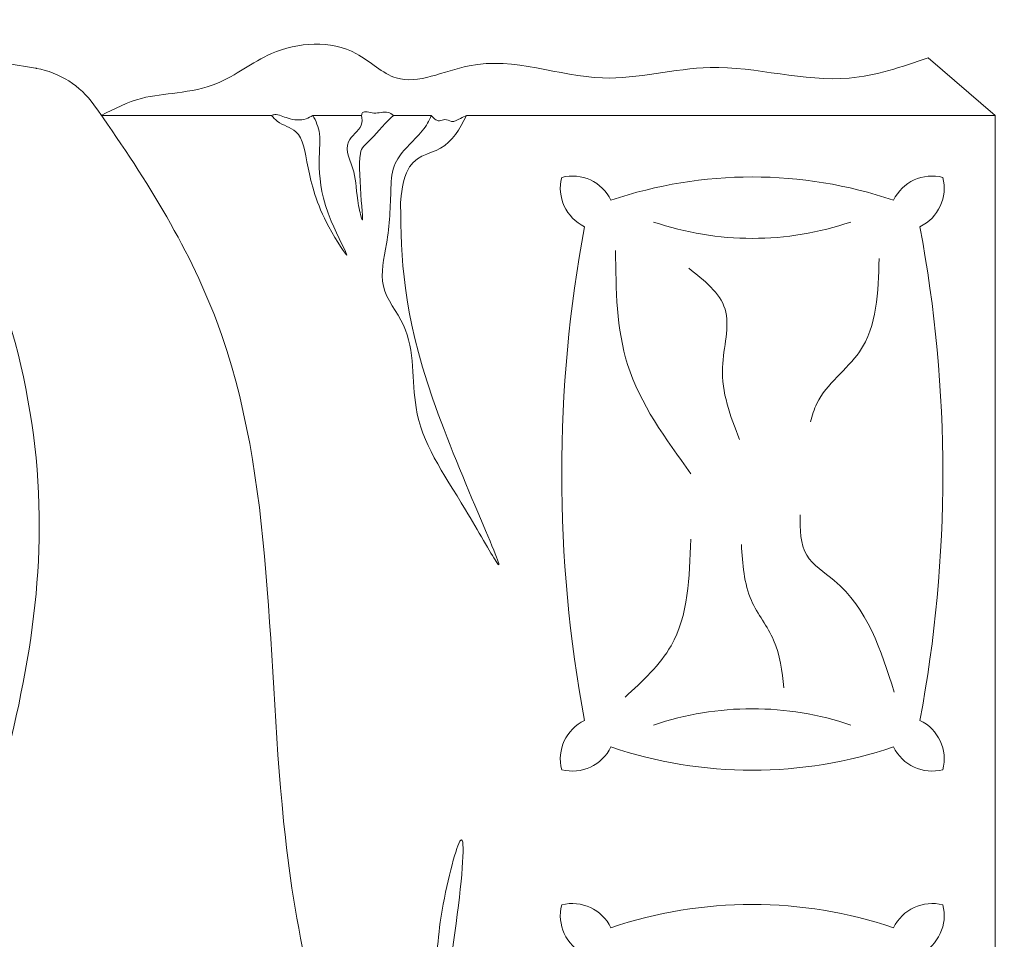
# Model space of a CAD drawing. Units: inches. Extents: x 2083 to 3317, y 1141 to 2115.
# Tile 242 of 256: x 3068 to 3108, y 1327 to 1365. Entities that reach past the tile are written whole.
import ezdxf

# ---------------------------------------------------------------- set-up
doc = ezdxf.new("R2010")
doc.units = ezdxf.units.IN
doc.layers.add('A-FURN', color=8, linetype='Continuous', lineweight=18)
doc.layers.add('www.cadblocksfree.com', color=7, linetype='Continuous', lineweight=9)
doc.layers.add('A-WALL-PATT', color=251, linetype='Continuous', lineweight=13, true_color=0x636466)

# ---------------------------------------------------------------- blocks, each defined once
blk = doc.blocks.new('bed')
at = {"layer": 'www.cadblocksfree.com', "ltscale": 0.2}
blk.add_line((3363.387, 1470.154), (3360.883, 1467.22), dxfattribs=at)
for points in [[(3426.379, 1449.413), (3426.379, 1470.154), (3363.387, 1470.154), (3363.387, 1447.076)], [(3363.387, 1445.539), (3363.387, 1443.892)], [(3363.387, 1442.495), (3363.387, 1440.369)], [(3363.387, 1438.564), (3363.387, 1431.137)]]:
    blk.add_lwpolyline(points, dxfattribs=at)
for centre, radius, start, end in [((3366.56, 1466.054), 1.87, 25.7901, 104.4834), ((3391.467, 1466.054), 1.87, 75.5166, 154.2099), ((3398.298, 1466.054), 1.87, 25.7901, 104.4834), ((3367.903, 1467.396), 1.87, 165.5166, 244.2099), ((3379.014, 1409.187), 58.677, 79.42346, 100.57654), ((3390.125, 1467.396), 1.87, 295.7901, 14.4834), ((3399.641, 1467.396), 1.87, 165.5166, 244.2099), ((3385.289, 1459.547), 19.215, 161.2852, 198.7148), ((3372.739, 1459.547), 19.215, 341.2852, 18.7148), ((3417.027, 1459.547), 19.215, 161.2852, 198.7148), ((3355.416, 1459.547), 13.338, 341.1598, 18.8402), ((3402.612, 1459.547), 13.338, 161.1598, 198.8402), ((3367.903, 1451.698), 1.87, 115.7901, 194.4834), ((3390.125, 1451.698), 1.87, 345.5166, 64.2099), ((3399.641, 1451.698), 1.87, 115.7901, 194.4834), ((3366.56, 1453.041), 1.87, 255.5166, 334.2099), ((3379.014, 1509.907), 58.677, 259.42346, 280.57654), ((3391.467, 1453.041), 1.87, 205.7901, 284.4834), ((3398.298, 1453.041), 1.87, 255.5166, 334.2099), ((3365.21, 1427.605), 3.937, 125.4209, 169.6982)]:
    blk.add_arc(centre, radius, start, end, dxfattribs=at)
for points, knots in [([(3360.883, 1467.22), (3361.272, 1466.08), (3362.328, 1462.983), (3360.73, 1458.154), (3362.389, 1452.621), (3360.35, 1448.139), (3362.429, 1444.241), (3360.039, 1441.931), (3360.256, 1438.678), (3362.05, 1436.545), (3362.42, 1434.517), (3362.566, 1432.758), (3363.096, 1431.712), (3363.387, 1431.137)], [0, 0, 0, 0, 3.550403, 9.643115, 14.356056, 20.206026, 23.427697, 25.46537, 29.172767, 31.884544, 33.668442, 35.237641, 37.145618, 37.145618, 37.145618, 37.145618]), ([(3388.545, 1465.744), (3386.719, 1465.161), (3384.357, 1464.407), (3382.678, 1461.635), (3381.454, 1461.638), (3380.813, 1461.64)], [0, 0, 0, 0, 5.530688, 7.154877, 8.940839, 8.940839, 8.940839, 8.940839]), ([(3369.625, 1465.083), (3371.104, 1465.041), (3373.625, 1464.969), (3375.264, 1462.52), (3376.483, 1462.165), (3376.755, 1462.086)], [0, 0, 0, 0, 4.163459, 7.093919, 7.934624, 7.934624, 7.934624, 7.934624]), ([(3388.358, 1460.927), (3387.639, 1460.846), (3386.254, 1460.689), (3384.483, 1459.224), (3382.96, 1459.127), (3382.112, 1459.073)], [0, 0, 0, 0, 2.127543, 4.10272, 6.58647, 6.58647, 6.58647, 6.58647]), ([(3370.049, 1456.774), (3370.592, 1457.459), (3371.713, 1458.876), (3374.682, 1457.893), (3376.505, 1458.594), (3377.525, 1458.985)], [0, 0, 0, 0, 2.388143, 4.935423, 8.166198, 8.166198, 8.166198, 8.166198]), ([(3369.287, 1453.579), (3370.996, 1453.599), (3374.587, 1453.639), (3377.497, 1455.762), (3379.021, 1456.874)], [0, 0, 0, 0, 5.002087, 10.507046, 10.507046, 10.507046, 10.507046]), ([(3388.77, 1453.995), (3388.068, 1454.761), (3386.268, 1456.726), (3383.544, 1456.811), (3381.881, 1456.863)], [0, 0, 0, 0, 3.013696, 7.735839, 7.735839, 7.735839, 7.735839]), ([(3367.269, 1444.201), (3369.575, 1444.23), (3373.917, 1444.284), (3385.471, 1449.8), (3379.558, 1446.493), (3376.808, 1444.477), (3372.948, 1444.924), (3370.926, 1443.14), (3368.771, 1443.702), (3367.359, 1443.752), (3366.554, 1443.781)], [0, 0, 0, 0, 8.61026, 16.221274, 18.843057, 23.804898, 27.440828, 29.356102, 31.203478, 33.650687, 33.650687, 33.650687, 33.650687]), ([(3409.943, 1443.853), (3408.469, 1444.451), (3404.443, 1446.042), (3391.397, 1447.599), (3398.64, 1445.767), (3402.973, 1445.759), (3406.219, 1444.095), (3408.408, 1442.961)], [0.0056315, 0.0056315, 0.0056315, 0.0056315, 0.1489731, 0.3882761, 0.4793617, 0.5593494, 0.7397317, 0.7397317, 0.7397317, 0.7397317]), ([(3363.387, 1447.076), (3363.429, 1446.99), (3363.529, 1446.784), (3363.731, 1446.461), (3363.506, 1446.154), (3363.665, 1445.905), (3363.559, 1445.673), (3363.444, 1445.584), (3363.387, 1445.539)], [0, 0, 0, 0, 0.293454, 0.701471, 1.003873, 1.254893, 1.47342, 1.69185, 1.69185, 1.69185, 1.69185]), ([(3363.387, 1447.076), (3363.991, 1446.782), (3365.084, 1446.124), (3365.119, 1444.371), (3367.129, 1444.191), (3367.269, 1444.201)], [0.0122268, 0.0122268, 0.0122268, 0.0122268, 0.0594721, 0.1062177, 0.134458, 0.134458, 0.134458, 0.134458]), ([(3366.554, 1443.781), (3366.17, 1443.775), (3365.174, 1443.901), (3364.4, 1444.957), (3363.626, 1445.461), (3363.387, 1445.539)], [0.15648839, 0.15648839, 0.15648839, 0.15648839, 0.18439755, 0.23137648, 0.25059846, 0.25059846, 0.25059846, 0.25059846]), ([(3363.387, 1443.892), (3363.335, 1443.815), (3363.165, 1443.56), (3363.346, 1443.124), (3363.233, 1442.791), (3363.225, 1442.533), (3363.341, 1442.506), (3363.387, 1442.495)], [0, 0, 0, 0, 0.27176, 0.887321, 1.189132, 1.388142, 1.515331, 1.515331, 1.515331, 1.515331]), ([(3363.387, 1443.892), (3363.631, 1443.61), (3364.671, 1442.733), (3364.886, 1442.149), (3369.073, 1442.744), (3366.773, 1442.243), (3365.832, 1442.298), (3364.615, 1441.552), (3363.961, 1442.542), (3363.537, 1442.524), (3363.387, 1442.495)], [0.0595743, 0.0595743, 0.0595743, 0.0595743, 0.0807529, 0.1037415, 0.1697201, 0.1760361, 0.2071372, 0.2404744, 0.2623409, 0.2736605, 0.2736605, 0.2736605, 0.2736605]), ([(3362.928, 1430.813), (3365.944, 1432.958), (3375.455, 1438.993), (3392.12, 1438.03), (3404.249, 1440.73), (3408.408, 1442.961)], [0.102872, 0.102872, 0.102872, 0.102872, 0.37972, 0.957702, 1.313793, 1.313793, 1.313793, 1.313793]), ([(3363.387, 1440.369), (3363.634, 1440.51), (3364.527, 1440.899), (3366.485, 1440.246), (3370.203, 1442.295), (3367.731, 1440.636), (3365.42, 1440.07), (3364.035, 1439.913), (3363.795, 1438.935), (3363.482, 1438.64), (3363.387, 1438.564)], [0.013856, 0.013856, 0.013856, 0.013856, 0.0348738, 0.0888667, 0.1078792, 0.1267378, 0.158714, 0.1937575, 0.2174868, 0.2267221, 0.2267221, 0.2267221, 0.2267221]), ([(3363.387, 1440.369), (3363.445, 1440.274), (3363.571, 1440.065), (3363.607, 1439.678), (3363.531, 1439.31), (3363.405, 1439.003), (3363.329, 1438.751), (3363.372, 1438.611), (3363.387, 1438.564)], [0, 0, 0, 0, 0.329977, 0.725302, 1.129072, 1.442831, 1.734218, 1.878348, 1.878348, 1.878348, 1.878348]), ([(3365.512, 1424.213), (3370.519, 1427.004), (3381.149, 1429.825), (3396.214, 1425.866), (3410.541, 1420.654), (3420.273, 1432.695), (3425.882, 1426.771), (3428.534, 1423.97)], [0.099185, 0.099185, 0.099185, 0.099185, 0.523647, 0.927087, 1.289918, 1.564439, 1.810555, 1.810555, 1.810555, 1.810555]), ([(3361.336, 1428.309), (3361.334, 1428.297), (3361.16, 1427.338), (3360.778, 1425.173), (3361.469, 1423.14), (3362.014, 1421.845)], [0.3128349, 0.3128349, 0.3128349, 0.3128349, 0.313751, 0.386958, 0.4759027, 0.4759027, 0.4759027, 0.4759027])]:
    blk.add_open_spline(points, degree=3, knots=knots, dxfattribs=at)

msp = doc.modelspace()

# ---------------------------------------------------------------- hatches: boundary and pattern name
at = {"layer": 'A-WALL-PATT'}
h = msp.add_hatch(color=256, dxfattribs=at)
h.dxf.hatch_style = 1
h.paths.add_polyline_path([(3126.96, 2020.761), (2748.96, 2020.761), (2604.96, 2020.761), (2226.96, 2020.761), (2226.96, 1702.761), (2466.96, 1702.761), (2466.96, 1582.761), (2418.96, 1582.761), (2418.96, 1477.761), (2226.96, 1477.761), (2226.96, 1263.261), (2544.96, 1263.261), (2544.96, 1411.761), (2604.96, 1411.761), (2685.96, 1411.761), (2685.96, 1420.761), (2604.96, 1420.761), (2604.96, 1573.761), (2604.96, 1702.761), (2604.96, 2011.761), (2748.96, 2011.761), (2748.96, 1702.761), (2862.96, 1702.761), (2862.96, 1621.761), (2871.96, 1621.761), (2871.96, 1702.761), (2883.96, 1702.761), (2883.96, 1706.939, -0.026459), (2883.96, 1711.761), (2757.96, 1711.761), (2757.96, 1807.761), (2787.96, 1807.761), (2787.96, 1812.261), (2757.96, 1812.261), (2757.96, 2011.761), (2877.96, 2011.761), (2877.96, 1812.261), (2847.96, 1812.261), (2847.96, 1807.761), (2889.836, 1807.761), (2889.836, 1812.261), (2882.46, 1812.261), (2882.46, 2011.761), (3117.96, 2011.761), (3117.96, 1812.261), (2937.836, 1812.261), (2937.836, 1807.761), (2995.71, 1807.761), (2995.71, 1796.118), (3000.21, 1796.118), (3000.21, 1807.761), (3117.96, 1807.761), (3117.96, 1711.761), (3000.21, 1711.761), (3000.21, 1760.118), (2998.573, 1760.118, -0.020711), (2995.71, 1760.118), (2995.71, 1711.761), (2931.96, 1711.761), (2931.96, 1702.761), (3126.96, 1702.761)])
h.paths.add_polyline_path([(2471.46, 2011.761), (2471.46, 1810.011), (2462.717, 1810.011), (2462.717, 1805.511), (2505.96, 1805.511), (2505.96, 1810.011), (2475.96, 1810.011), (2475.96, 2011.761), (2595.96, 2011.761), (2595.96, 1810.011), (2565.96, 1810.011), (2565.96, 1805.511), (2595.96, 1805.511), (2595.96, 1711.761), (2235.96, 1711.761), (2235.96, 1805.511), (2353.71, 1805.511), (2353.71, 1796.054), (2358.21, 1796.054), (2358.21, 1805.511), (2414.717, 1805.511), (2414.717, 1810.011), (2235.96, 1810.011), (2235.96, 2011.761)], flags=16)
h.paths.add_polyline_path([(2270.205, 1994.61), (2270.205, 1970.61), (2246.205, 1970.61), (2246.205, 1994.61)], flags=0)
edge = h.paths.add_edge_path(flags=0)
edge.add_ellipse((2332.027, 1899.798), major_axis=(-3.043, 3.043), ratio=0.168252, start_angle=-161.3322, end_angle=-156.3071, ccw=False)
edge.add_ellipse((2333.082, 1898.744), major_axis=(-1.055, 1.055), ratio=0.453532, start_angle=-123.371, end_angle=-94.1591)
edge = h.paths.add_edge_path(flags=0)
edge.add_ellipse((2332.027, 1968.876), major_axis=(3.043, 3.043), ratio=0.168252, start_angle=18.6678, end_angle=23.6929)
edge.add_spline(control_points=[(2332.926, 1970.691), (2332.227, 1970.336), (2330.894, 1969.659), (2328.413, 1970.932), (2327.204, 1967.749), (2324.71, 1969.956), (2322.533, 1967.012), (2320.013, 1971.296), (2317.68, 1968.158), (2316.041, 1967.102), (2315.427, 1966.81)], knot_values=[0, 0, 0, 0, 2.267059, 4.324559, 6.685584, 8.878641, 11.121502, 14.300359, 17.755284, 19.732645, 19.732645, 19.732645, 19.732645], degree=3, periodic=0)
edge.add_ellipse((2332.027, 1968.876), major_axis=(3.043, 3.043), ratio=0.168252, start_angle=18.6678, end_angle=23.6929, ccw=False)
edge.add_ellipse((2333.082, 1969.931), major_axis=(1.055, 1.055), ratio=0.453532, start_angle=56.629, end_angle=85.8409, ccw=False)
edge = h.paths.add_edge_path(flags=0)
edge.add_spline(control_points=[(2296.428, 1967.988), (2293.628, 1965.336), (2287.704, 1959.727), (2299.744, 1949.996), (2294.533, 1935.669), (2290.573, 1920.604), (2293.394, 1909.974), (2296.185, 1904.967)], knot_values=[0.099185, 0.099185, 0.099185, 0.099185, 0.345301, 0.619822, 0.982653, 1.386093, 1.810555, 1.810555, 1.810555, 1.810555], degree=3, periodic=0)
edge.add_spline(control_points=[(2296.185, 1904.967), (2297.384, 1902.619), (2298.001, 1901.949), (2298.553, 1901.468)], knot_values=[0.006246, 0.006246, 0.006246, 0.006246, 0.055476, 0.055476, 0.055476, 0.055476], degree=3, periodic=0)
edge.add_spline(control_points=[(2298.553, 1901.468), (2297.259, 1900.923), (2295.225, 1900.232), (2293.06, 1900.614), (2292.101, 1900.788), (2292.09, 1900.791)], knot_values=[0.312835, 0.312835, 0.312835, 0.312835, 0.40178, 0.474987, 0.475903, 0.475903, 0.475903, 0.475903], degree=3, periodic=0)
edge.add_arc((2292.794, 1904.664), 3.937, 215.4209, 259.6982, ccw=False)
edge.add_spline(control_points=[(2289.585, 1902.382), (2289.477, 1902.535), (2289.368, 1902.688), (2289.261, 1902.841)], knot_values=[0.102872, 0.102872, 0.102872, 0.102872, 0.116896, 0.116896, 0.116896, 0.116896], degree=3, periodic=0)
edge.add_spline(control_points=[(2289.261, 1902.841), (2288.687, 1902.55), (2287.64, 1902.02), (2285.881, 1901.874), (2283.853, 1901.504), (2281.72, 1899.711), (2278.467, 1899.493), (2276.157, 1901.883), (2272.259, 1899.804), (2267.778, 1901.843), (2262.244, 1900.184), (2257.415, 1901.782), (2254.318, 1900.726), (2253.178, 1900.337)], knot_values=[0, 0, 0, 0, 1.907977, 3.477176, 5.261074, 7.972851, 11.680248, 13.717921, 16.939592, 22.789562, 27.502503, 33.595215, 37.145618, 37.145618, 37.145618, 37.145618], degree=3, periodic=0)
edge.add_line((2253.178, 1900.337), (2250.244, 1902.841))
edge.add_line((2250.244, 1902.841), (2250.244, 1965.833))
edge.add_line((2250.244, 1965.833), (2253.178, 1968.337))
edge.add_spline(control_points=[(2253.178, 1968.337), (2254.318, 1967.948), (2257.415, 1966.892), (2262.244, 1968.49), (2267.778, 1966.831), (2271.527, 1968.537), (2273.876, 1967.828), (2274.207, 1967.728)], knot_values=[0, 0, 0, 0, 0.09018, 0.244935, 0.364644, 0.513233, 0.537855, 0.537855, 0.537855, 0.537855], degree=3, periodic=0)
edge.add_arc((2274.353, 1963.793), 3.937, 72.0511, 92.1279, ccw=False)
edge.add_arc((2281.297, 1985.23), 18.596, 252.0511, 288.5657)
edge.add_arc((2292.317, 1956.029), 12.646, 71.0268, 113.7782, ccw=False)
edge = h.paths.add_edge_path(flags=0)
edge.add_spline(control_points=[(2274.899, 1951.856), (2275.066, 1951.617), (2275.233, 1951.377), (2275.398, 1951.136)], knot_values=[1.409916, 1.409916, 1.409916, 1.409916, 1.43159, 1.43159, 1.43159, 1.43159], degree=3, periodic=0)
edge.add_spline(control_points=[(2275.398, 1951.136), (2275.792, 1950.562), (2276.179, 1949.984), (2276.546, 1949.397)], knot_values=[1.358238, 1.358238, 1.358238, 1.358238, 1.409916, 1.409916, 1.409916, 1.409916], degree=3, periodic=0)
edge.add_line((2276.546, 1949.397), (2277.437, 1947.862))
edge.add_spline(control_points=[(2277.437, 1947.862), (2276.304, 1945.673), (2274.64, 1942.427), (2274.632, 1938.094), (2272.799, 1930.852), (2274.356, 1943.897), (2275.948, 1947.923), (2276.546, 1949.397)], knot_values=[0.005632, 0.005632, 0.005632, 0.005632, 0.186014, 0.266002, 0.357087, 0.59639, 0.739732, 0.739732, 0.739732, 0.739732], degree=3, periodic=0)
edge.add_spline(control_points=[(2276.546, 1949.397), (2276.179, 1949.984), (2275.792, 1950.562), (2275.398, 1951.136)], knot_values=[1.358238, 1.358238, 1.358238, 1.358238, 1.409916, 1.409916, 1.409916, 1.409916], degree=3, periodic=0)
edge.add_spline(control_points=[(2275.398, 1951.136), (2274.943, 1950.08), (2274.208, 1948.025), (2273.935, 1944.851), (2272.469, 1937.627), (2273.466, 1945.696), (2274.701, 1951.059), (2274.899, 1951.856)], knot_values=[0.104364, 0.104364, 0.104364, 0.104364, 0.189636, 0.269624, 0.36071, 0.600013, 0.644622, 0.644622, 0.644622, 0.644622], degree=3, periodic=0)
h.paths.add_polyline_path([(2269.168, 1963.128, -0.357527), (2268.171, 1960.976, -0.092561), (2268.171, 1939.436, -0.357527), (2269.168, 1937.285, -0.357527), (2267.016, 1938.282, -0.164785), (2254.686, 1938.282, -0.357527), (2252.534, 1937.285, -0.357527), (2253.531, 1939.436, -0.092561), (2253.531, 1960.976, -0.357527), (2252.534, 1963.128, -0.357527), (2254.686, 1962.131, -0.164785), (2267.016, 1962.131, -0.357527)], flags=0)
h.paths.add_polyline_path([(2248.874, 1967.802), (2248.874, 1957.028), (2249.458, 1957.028), (2249.458, 1911.647), (2248.874, 1911.647), (2248.874, 1900.873), (2246.512, 1900.873, 0.197327), (2244.15, 1902.457), (2244.15, 1966.218, 0.197327), (2246.512, 1967.802)], flags=0)
h.paths.add_polyline_path([(2269.168, 1931.389, -0.357527), (2268.171, 1929.238, -0.092561), (2268.171, 1907.698, -0.357527), (2269.168, 1905.547, -0.357527), (2267.016, 1906.544, -0.164785), (2254.686, 1906.544, -0.357527), (2252.534, 1905.547, -0.357527), (2253.531, 1907.698, -0.092561), (2253.531, 1929.238, -0.357527), (2252.534, 1931.389, -0.357527), (2254.686, 1930.392, -0.164785), (2267.016, 1930.392, -0.357527)], flags=0)
edge = h.paths.add_edge_path(flags=0)
edge.add_spline(control_points=[(2276.197, 1906.724), (2276.168, 1909.029), (2276.114, 1913.372), (2270.598, 1924.925), (2273.905, 1919.013), (2275.922, 1916.262), (2275.475, 1912.402), (2277.258, 1910.381), (2276.696, 1908.225), (2276.646, 1906.813), (2276.618, 1906.008)], knot_values=[0, 0, 0, 0, 8.61026, 16.221274, 18.843057, 23.804898, 27.440828, 29.356102, 31.203478, 33.650687, 33.650687, 33.650687, 33.650687], degree=3, periodic=0)
edge.add_spline(control_points=[(2276.618, 1906.008), (2276.623, 1905.624), (2276.498, 1904.629), (2275.442, 1903.855), (2274.937, 1903.08), (2274.859, 1902.841)], knot_values=[0.156488, 0.156488, 0.156488, 0.156488, 0.184398, 0.231376, 0.250598, 0.250598, 0.250598, 0.250598], degree=3, periodic=0)
edge.add_line((2274.859, 1902.841), (2276.506, 1902.841))
edge.add_spline(control_points=[(2276.506, 1902.841), (2276.788, 1903.085), (2277.665, 1904.125), (2278.25, 1904.341), (2277.654, 1908.527), (2278.156, 1906.228), (2278.1, 1905.286), (2278.847, 1904.069), (2277.857, 1903.415), (2277.874, 1902.991), (2277.904, 1902.841)], knot_values=[0.059574, 0.059574, 0.059574, 0.059574, 0.080753, 0.103741, 0.16972, 0.176036, 0.207137, 0.240474, 0.262341, 0.27366, 0.27366, 0.27366, 0.27366], degree=3, periodic=0)
edge.add_line((2277.904, 1902.841), (2280.03, 1902.841))
edge.add_spline(control_points=[(2280.03, 1902.841), (2279.888, 1903.088), (2279.499, 1903.982), (2280.152, 1905.939), (2278.104, 1909.658), (2279.762, 1907.185), (2280.328, 1904.875), (2280.485, 1903.49), (2281.463, 1903.249), (2281.758, 1902.936), (2281.834, 1902.841)], knot_values=[0.013856, 0.013856, 0.013856, 0.013856, 0.034874, 0.088867, 0.107879, 0.126738, 0.158714, 0.193757, 0.217487, 0.226722, 0.226722, 0.226722, 0.226722], degree=3, periodic=0)
edge.add_spline(control_points=[(2281.834, 1902.841), (2281.788, 1902.827), (2281.647, 1902.783), (2281.396, 1902.859), (2281.088, 1902.985), (2280.721, 1903.061), (2280.333, 1903.026), (2280.125, 1902.899), (2280.03, 1902.841)], knot_values=[0, 0, 0, 0, 0.14413, 0.435517, 0.749276, 1.153046, 1.548371, 1.878348, 1.878348, 1.878348, 1.878348], degree=3, periodic=0)
edge.add_line((2280.03, 1902.841), (2277.904, 1902.841))
edge.add_spline(control_points=[(2277.904, 1902.841), (2277.893, 1902.796), (2277.865, 1902.68), (2277.607, 1902.687), (2277.274, 1902.801), (2276.838, 1902.62), (2276.584, 1902.789), (2276.506, 1902.841)], knot_values=[0, 0, 0, 0, 0.127189, 0.326199, 0.628009, 1.24357, 1.515331, 1.515331, 1.515331, 1.515331], degree=3, periodic=0)
edge.add_line((2276.506, 1902.841), (2274.859, 1902.841))
edge.add_spline(control_points=[(2274.859, 1902.841), (2274.814, 1902.899), (2274.725, 1903.013), (2274.493, 1903.119), (2274.244, 1902.961), (2273.937, 1903.185), (2273.614, 1902.983), (2273.408, 1902.883), (2273.322, 1902.841)], knot_values=[0, 0, 0, 0, 0.21843, 0.436957, 0.687977, 0.990379, 1.398396, 1.69185, 1.69185, 1.69185, 1.69185], degree=3, periodic=0)
edge.add_spline(control_points=[(2273.322, 1902.841), (2273.617, 1903.446), (2274.274, 1904.538), (2276.027, 1904.574), (2276.207, 1906.584), (2276.197, 1906.724)], knot_values=[0.012227, 0.012227, 0.012227, 0.012227, 0.059472, 0.106218, 0.134458, 0.134458, 0.134458, 0.134458], degree=3, periodic=0)
h.paths.add_polyline_path([(2270.776, 1897.79), (2270.776, 1873.79), (2246.776, 1873.79), (2246.776, 1897.79)], flags=0)
h.paths.add_polyline_path([(2353.71, 1760.005), (2353.71, 1760.054), (2358.21, 1760.054, -0.033729)], flags=0)
h.paths.add_polyline_path([(2321.819, 1737.529), (2341.995, 1737.529, -0.414214), (2343.203, 1736.321), (2343.203, 1721.021, -0.414214), (2341.995, 1719.813), (2321.819, 1719.813, -0.414214), (2320.611, 1721.021), (2320.611, 1736.321, -0.414214)], flags=0)
h.paths.add_polyline_path([(2324.235, 1736.321), (2339.579, 1736.321, -0.414214), (2341.995, 1733.905), (2341.995, 1725.45, -0.414214), (2339.579, 1723.034), (2333.681, 1723.034), (2333.845, 1722.045, -0.870646), (2335.425, 1721.826, -0.767327), (2333.923, 1721.423), (2331.291, 1721.423, -0.767327), (2329.788, 1721.826, -0.870646), (2331.368, 1722.045), (2331.533, 1723.034), (2324.235, 1723.034, -0.414214), (2321.819, 1725.45), (2321.819, 1733.905, -0.414214)], flags=0)
h.paths.add_polyline_path([(2570.484, 1928.615), (2589.684, 1928.615), (2590.169, 1928.615), (2590.169, 1904.993), (2570.484, 1904.993)], flags=0)
h.paths.add_polyline_path([(2574.447, 1927.264, -1), (2572.829, 1927.264, -1)], flags=0)
h.paths.add_polyline_path([(2573.09, 1926.941), (2573.925, 1927.776), (2574.148, 1927.553), (2573.313, 1926.718)], flags=0)
h.paths.add_polyline_path([(2578.779, 1919.73, -1), (2571.592, 1919.73, -1)], flags=0)
h.paths.add_polyline_path([(2578.385, 1919.73, -1), (2571.985, 1919.73, -1)], flags=0)
h.paths.add_polyline_path([(2331.596, 1729.476, -1), (2333.618, 1729.476, -1)], flags=0)
h.paths.add_polyline_path([(2578.034, 1927.264, -1), (2576.416, 1927.264, -1)], flags=0)
h.paths.add_polyline_path([(2576.689, 1927.531), (2576.912, 1927.754), (2577.747, 1926.919), (2577.524, 1926.696)], flags=0)
h.paths.add_polyline_path([(2578.139, 1909.86, -1), (2572.232, 1909.86, -1)], flags=0)
h.paths.add_polyline_path([(2577.745, 1909.86, -1), (2572.625, 1909.86, -1)], flags=0)
h.paths.add_polyline_path([(2583.798, 1927.264, -1), (2582.179, 1927.264, -1)], flags=0)
h.paths.add_polyline_path([(2582.719, 1927.754), (2583.554, 1926.919), (2583.331, 1926.696), (2582.496, 1927.531)], flags=0)
h.paths.add_polyline_path([(2582.496, 1927.531), (2582.719, 1927.754), (2583.554, 1926.919), (2583.331, 1926.696)], flags=0)
h.paths.add_polyline_path([(2587.739, 1920.53, -1), (2581.832, 1920.53, -1)], flags=0)
h.paths.add_polyline_path([(2587.345, 1920.53, -1), (2582.225, 1920.53, -1)], flags=0)
h.paths.add_polyline_path([(2587.385, 1927.264, -1), (2585.766, 1927.264, -1)], flags=0)
h.paths.add_polyline_path([(2586.082, 1926.98), (2586.917, 1927.815), (2587.14, 1927.593), (2586.305, 1926.758)], flags=0)
h.paths.add_polyline_path([(2588.379, 1910.66, -1), (2581.192, 1910.66, -1)], flags=0)
h.paths.add_polyline_path([(2587.985, 1910.66, -1), (2581.585, 1910.66, -1)], flags=0)
h.paths.add_polyline_path([(2417.168, 1729.478), (2437.344, 1729.478, -0.414214), (2438.552, 1728.27), (2438.552, 1712.969, -0.414214), (2437.344, 1711.761), (2417.168, 1711.761, -0.414214), (2415.96, 1712.969), (2415.96, 1728.27, -0.414214)], flags=0)
h.paths.add_polyline_path([(2419.584, 1728.27), (2434.928, 1728.27, -0.414214), (2437.344, 1725.854), (2437.344, 1717.398, -0.414214), (2434.928, 1714.983), (2429.029, 1714.983), (2429.194, 1713.994, -0.870646), (2430.774, 1713.775, -0.767327), (2429.271, 1713.372), (2426.64, 1713.372, -0.767327), (2425.137, 1713.775, -0.870646), (2426.717, 1713.994), (2426.882, 1714.983), (2419.584, 1714.983, -0.414214), (2417.168, 1717.398), (2417.168, 1725.854, -0.414214)], flags=0)
h.paths.add_polyline_path([(2419.584, 1728.27), (2434.928, 1728.27, -0.414214), (2437.344, 1725.854), (2437.344, 1717.398, -0.414214), (2434.928, 1714.983), (2429.029, 1714.983), (2428.358, 1719.009), (2427.553, 1719.009), (2426.882, 1714.983), (2419.584, 1714.983, -0.414214), (2417.168, 1717.398), (2417.168, 1725.854, -0.414214)], flags=0)
h.paths.add_polyline_path([(2426.944, 1721.425, -1), (2428.967, 1721.425, -1)], flags=0)
h.paths.add_polyline_path([(2475.96, 1702.761), (2595.96, 1702.761), (2595.96, 1582.761), (2475.96, 1582.761)], flags=16)
h.paths.add_polyline_path([(2427.96, 1573.761), (2595.96, 1573.761), (2595.96, 1468.761), (2595.96, 1420.761), (2384.46, 1420.761), (2384.46, 1468.761), (2427.96, 1468.761)], flags=16)
h.paths.add_polyline_path([(2379.96, 1468.761), (2379.96, 1420.761), (2235.96, 1420.761), (2235.96, 1468.761)], flags=16)
h.paths.add_polyline_path([(2317.816, 1466.696), (2337.992, 1466.696, -0.414214), (2339.2, 1465.488), (2339.2, 1450.187, -0.414214), (2337.992, 1448.979), (2317.816, 1448.979, -0.414214), (2316.608, 1450.187), (2316.608, 1465.488, -0.414214)], flags=0)
h.paths.add_polyline_path([(2320.232, 1465.488), (2335.576, 1465.488, -0.414214), (2337.992, 1463.072), (2337.992, 1454.616, -0.414214), (2335.576, 1452.2), (2329.677, 1452.2), (2329.842, 1451.212, -0.870646), (2331.422, 1450.992, -0.767327), (2329.92, 1450.59), (2327.288, 1450.59, -0.767327), (2325.785, 1450.992, -0.870646), (2327.365, 1451.212), (2327.53, 1452.2), (2320.232, 1452.2, -0.414214), (2317.816, 1454.616), (2317.816, 1463.072, -0.414214)], flags=0)
h.paths.add_polyline_path([(2320.232, 1465.488), (2335.576, 1465.488, -0.414214), (2337.992, 1463.072), (2337.992, 1454.616, -0.414214), (2335.576, 1452.2), (2329.677, 1452.2), (2329.006, 1456.227), (2328.201, 1456.227), (2327.53, 1452.2), (2320.232, 1452.2, -0.414214), (2317.816, 1454.616), (2317.816, 1463.072, -0.414214)], flags=0)
h.paths.add_polyline_path([(2327.593, 1458.643, -1), (2329.615, 1458.643, -1)], flags=0)
h.paths.add_polyline_path([(2244.412, 1433.34), (2241.921, 1433.34, -0.414214), (2240.018, 1435.244), (2240.018, 1440.953, -0.414211), (2241.921, 1442.856), (2244.412, 1442.856, -1.976472)], flags=0)
h.paths.add_polyline_path([(2245.357, 1434.398, -0.414214), (2245.357, 1441.799, -2.144098)], flags=0)
h.paths.add_polyline_path([(2535.96, 1416.261), (2535.96, 1272.261), (2235.96, 1272.261), (2235.96, 1416.261)], flags=16)
h.paths.add_polyline_path([(2260.12, 1384.293), (2260.12, 1362.039), (2237.865, 1362.039), (2237.865, 1384.293)], flags=0)
edge = h.paths.add_edge_path(flags=0)
edge.add_line((2318.252, 1362.093), (2318.146, 1362.001))
edge.add_ellipse((2317.445, 1360.431), major_axis=(2.822, 2.822), ratio=0.168252, start_angle=18.6678, end_angle=20.9481, ccw=False)
edge.add_ellipse((2318.423, 1361.409), major_axis=(0.978, 0.978), ratio=0.453532, start_angle=56.629, end_angle=70.2262, ccw=False)
edge = h.paths.add_edge_path(flags=0)
edge.add_line((2319.107, 1295.571), (2319.015, 1295.677))
edge.add_ellipse((2317.445, 1296.378), major_axis=(-2.822, 2.822), ratio=0.168252, start_angle=-161.3322, end_angle=-159.0519, ccw=False)
edge.add_ellipse((2318.423, 1295.4), major_axis=(-0.978, 0.978), ratio=0.453532, start_angle=-123.371, end_angle=-109.7738)
edge = h.paths.add_edge_path(flags=0)
edge.add_spline(control_points=[(2284.21, 1301.17), (2284.581, 1300.445), (2284.891, 1299.892), (2285.16, 1299.461)], knot_values=[0.039066, 0.039066, 0.039066, 0.039066, 0.055476, 0.055476, 0.055476, 0.055476], degree=3, periodic=0)
edge.add_line((2285.16, 1299.461), (2284.21, 1301.17))
edge = h.paths.add_edge_path(flags=0)
edge.add_line((2280.412, 1297.298), (2283.37, 1297.036))
edge.add_line((2283.37, 1297.036), (2286.406, 1297.926))
edge.add_spline(control_points=[(2286.406, 1297.926), (2285.305, 1297.463), (2284.345, 1297.129), (2283.37, 1297.036)], knot_values=[0.394369, 0.394369, 0.394369, 0.394369, 0.475903, 0.475903, 0.475903, 0.475903], degree=3, periodic=0)
edge.add_spline(control_points=[(2283.37, 1297.036), (2283.281, 1297.028), (2282.316, 1296.957), (2281.313, 1297.134), (2280.423, 1297.296), (2280.412, 1297.298)], knot_values=[0.312835, 0.312835, 0.312835, 0.312835, 0.320246, 0.393453, 0.394369, 0.394369, 0.394369, 0.394369], degree=3, periodic=0)
edge = h.paths.add_edge_path(flags=0)
edge.add_line((2284.436, 1359.607), (2280.446, 1355.328))
edge.add_line((2280.446, 1355.328), (2279.58, 1351.018))
edge.add_line((2279.58, 1351.018), (2282.413, 1346.58))
edge.add_spline(control_points=[(2282.413, 1346.58), (2283.153, 1345.589), (2284.253, 1344.029), (2284.801, 1342.387), (2284.935, 1341.806)], knot_values=[1.240098, 1.240098, 1.240098, 1.240098, 1.332892, 1.382712, 1.382712, 1.382712, 1.382712], degree=3, periodic=0)
edge.add_spline(control_points=[(2284.935, 1341.806), (2285.319, 1340.141), (2285.233, 1338.409), (2284.91, 1336.654)], knot_values=[1.097484, 1.097484, 1.097484, 1.097484, 1.240098, 1.240098, 1.240098, 1.240098], degree=3, periodic=0)
edge.add_spline(control_points=[(2284.91, 1336.654), (2284.587, 1334.899), (2284.027, 1333.12), (2283.463, 1331.361)], knot_values=[0.95487, 0.95487, 0.95487, 0.95487, 1.097484, 1.097484, 1.097484, 1.097484], degree=3, periodic=0)
edge.add_line((2283.463, 1331.361), (2281.89, 1326.153))
edge.add_line((2281.89, 1326.153), (2280.756, 1321.056))
edge.add_line((2280.756, 1321.056), (2280.299, 1316.002))
edge.add_line((2280.299, 1316.002), (2280.716, 1310.95))
edge.add_line((2280.716, 1310.95), (2282.028, 1305.972))
edge.add_line((2282.028, 1305.972), (2284.21, 1301.17))
edge.add_spline(control_points=[(2284.21, 1301.17), (2283.341, 1302.73), (2282.612, 1304.336), (2282.028, 1305.972)], knot_values=[0.099185, 0.099185, 0.099185, 0.099185, 0.241799, 0.241799, 0.241799, 0.241799], degree=3, periodic=0)
edge.add_spline(control_points=[(2282.028, 1305.972), (2281.444, 1307.608), (2281.005, 1309.273), (2280.716, 1310.95)], knot_values=[0.241799, 0.241799, 0.241799, 0.241799, 0.384413, 0.384413, 0.384413, 0.384413], degree=3, periodic=0)
edge.add_spline(control_points=[(2280.716, 1310.95), (2280.433, 1312.588), (2280.289, 1314.277), (2280.299, 1315.962), (2280.299, 1316.002)], knot_values=[0.384413, 0.384413, 0.384413, 0.384413, 0.523647, 0.527028, 0.527028, 0.527028, 0.527028], degree=3, periodic=0)
edge.add_spline(control_points=[(2280.299, 1316.002), (2280.312, 1317.687), (2280.478, 1319.368), (2280.756, 1321.056)], knot_values=[0.527028, 0.527028, 0.527028, 0.527028, 0.669642, 0.669642, 0.669642, 0.669642], degree=3, periodic=0)
edge.add_spline(control_points=[(2280.756, 1321.056), (2281.035, 1322.744), (2281.426, 1324.44), (2281.89, 1326.153)], knot_values=[0.669642, 0.669642, 0.669642, 0.669642, 0.812256, 0.812256, 0.812256, 0.812256], degree=3, periodic=0)
edge.add_spline(control_points=[(2281.89, 1326.153), (2282.264, 1327.533), (2282.788, 1329.262), (2283.353, 1331.018), (2283.463, 1331.361)], knot_values=[0.812256, 0.812256, 0.812256, 0.812256, 0.927087, 0.95487, 0.95487, 0.95487, 0.95487], degree=3, periodic=0)
edge.add_line((2283.463, 1331.361), (2284.91, 1336.654))
edge.add_line((2284.91, 1336.654), (2284.935, 1341.806))
edge.add_line((2284.935, 1341.806), (2282.413, 1346.58))
edge.add_spline(control_points=[(2282.413, 1346.58), (2281.275, 1348.104), (2280.078, 1349.57), (2279.58, 1351.018)], knot_values=[1.382712, 1.382712, 1.382712, 1.382712, 1.525326, 1.525326, 1.525326, 1.525326], degree=3, periodic=0)
edge.add_spline(control_points=[(2279.58, 1351.018), (2279.443, 1351.415), (2279.136, 1352.857), (2279.735, 1354.29), (2280.446, 1355.328)], knot_values=[1.525326, 1.525326, 1.525326, 1.525326, 1.564439, 1.667941, 1.667941, 1.667941, 1.667941], degree=3, periodic=0)
edge.add_spline(control_points=[(2280.446, 1355.328), (2281.426, 1356.758), (2282.931, 1358.183), (2284.436, 1359.607)], knot_values=[1.667941, 1.667941, 1.667941, 1.667941, 1.810555, 1.810555, 1.810555, 1.810555], degree=3, periodic=0)
edge.add_arc((2280.623, 1348.518), 11.726, 71.0268, 113.7782)
edge.add_arc((2270.405, 1375.595), 17.244, 252.0511, 288.5657, ccw=False)
edge.add_arc((2263.966, 1355.718), 3.651, 72.0511, 92.1279)
edge.add_arc((2263.966, 1355.718), 3.651, 92.1279, 177.9851)
edge.add_spline(control_points=[(2260.318, 1355.846), (2260.26, 1354.221), (2260.551, 1350.187), (2262.999, 1346.766), (2264.473, 1344.649)], knot_values=[1.43159, 1.43159, 1.43159, 1.43159, 1.564144, 1.770695, 1.770695, 1.770695, 1.770695], degree=3, periodic=0)
edge.add_line((2264.473, 1344.649), (2264.936, 1343.983))
edge.add_spline(control_points=[(2263.801, 1340.248), (2263.843, 1340.514), (2264.067, 1341.756), (2264.513, 1343.002), (2264.935, 1343.981)], knot_values=[0.53657, 0.53657, 0.53657, 0.53657, 0.559349, 0.644622, 0.644622, 0.644622, 0.644622], degree=3, periodic=0)
edge.add_spline(control_points=[(2264.935, 1343.981), (2265.118, 1343.715), (2265.299, 1343.448), (2265.477, 1343.179)], knot_values=[1.384077, 1.384077, 1.384077, 1.384077, 1.409916, 1.409916, 1.409916, 1.409916], degree=3, periodic=0)
edge.add_spline(control_points=[(2265.477, 1343.179), (2265.655, 1342.911), (2265.829, 1342.641), (2265.999, 1342.369)], knot_values=[1.358238, 1.358238, 1.358238, 1.358238, 1.384077, 1.384077, 1.384077, 1.384077], degree=3, periodic=0)
edge.add_line((2265.999, 1342.369), (2266.826, 1340.946))
edge.add_spline(control_points=[(2266.826, 1340.946), (2268.894, 1337.09), (2271.398, 1325.843), (2270.516, 1310.569), (2275.919, 1301.861), (2277.79, 1299.199)], knot_values=[0.116896, 0.116896, 0.116896, 0.116896, 0.472987, 1.050969, 1.313793, 1.313793, 1.313793, 1.313793], degree=3, periodic=0)
edge.add_spline(control_points=[(2277.79, 1299.199), (2277.839, 1299.128), (2277.889, 1299.057), (2277.94, 1298.987)], knot_values=[0.109884, 0.109884, 0.109884, 0.109884, 0.116896, 0.116896, 0.116896, 0.116896], degree=3, periodic=0)
edge.add_line((2277.94, 1298.987), (2277.789, 1299.199))
edge.add_spline(control_points=[(2277.789, 1299.199), (2277.257, 1298.929), (2276.286, 1298.438), (2275.039, 1298.334), (2274.383, 1298.239), (2274.215, 1298.209)], knot_values=[33.12187, 33.12187, 33.12187, 33.12187, 35.029056, 36.598255, 37.144827, 37.144827, 37.144827, 37.144827], degree=3, periodic=0)
edge.add_line((2274.215, 1298.209), (2273.073, 1297.893))
edge.add_spline(control_points=[(2273.073, 1297.893), (2272.323, 1297.58), (2271.039, 1296.511), (2269.248, 1296.226), (2268.423, 1296.375)], knot_values=[26.532584, 26.532584, 26.532584, 26.532584, 29.198919, 31.839101, 31.839101, 31.839101, 31.839101], degree=3, periodic=0)
edge.add_line((2268.423, 1296.375), (2263.879, 1297.458))
edge.add_spline(control_points=[(2263.879, 1297.458), (2263.556, 1297.359), (2261.86, 1296.839), (2260.239, 1297.282), (2258.933, 1297.516)], knot_values=[15.919551, 15.919551, 15.919551, 15.919551, 16.939592, 21.226067, 21.226067, 21.226067, 21.226067], degree=3, periodic=0)
edge.add_line((2258.933, 1297.516), (2254.055, 1297.329))
edge.add_spline(control_points=[(2254.055, 1297.329), (2253.756, 1297.296), (2252.114, 1297.165), (2250.462, 1297.544), (2249.13, 1297.668)], knot_values=[5.306517, 5.306517, 5.306517, 5.306517, 6.276435, 10.613034, 10.613034, 10.613034, 10.613034], degree=3, periodic=0)
edge.add_line((2249.13, 1297.668), (2244.332, 1296.878))
edge.add_line((2244.332, 1296.878), (2241.611, 1299.199))
edge.add_line((2241.611, 1299.199), (2241.611, 1357.609))
edge.add_line((2241.611, 1357.609), (2244.332, 1359.931))
edge.add_line((2244.332, 1359.931), (2252.729, 1359.543))
edge.add_spline(control_points=[(2252.729, 1359.543), (2252.871, 1359.546), (2253.306, 1359.548), (2253.74, 1359.514), (2254.032, 1359.482)], knot_values=[0.233291, 0.233291, 0.233291, 0.233291, 0.244935, 0.268927, 0.268927, 0.268927, 0.268927], degree=3, periodic=0)
edge.add_line((2254.032, 1359.482), (2259.587, 1359.416))
edge.add_spline(control_points=[(2259.587, 1359.416), (2260.677, 1359.629), (2262.073, 1359.897), (2263.524, 1359.459), (2263.83, 1359.366)], knot_values=[0.422516, 0.422516, 0.422516, 0.422516, 0.513233, 0.537855, 0.537855, 0.537855, 0.537855], degree=3, periodic=0)
edge.add_arc((2263.966, 1355.718), 3.651, 72.0511, 92.1279, ccw=False)
edge.add_arc((2270.405, 1375.595), 17.244, 252.0511, 288.5657)
edge.add_arc((2280.623, 1348.518), 11.726, 71.0268, 113.7782, ccw=False)
h.paths.add_polyline_path([(2240.341, 1359.435), (2240.341, 1349.444), (2240.882, 1349.444), (2240.882, 1307.365), (2240.341, 1307.365), (2240.341, 1297.374), (2238.15, 1297.374, 0.197327), (2235.96, 1298.843), (2235.96, 1357.966, 0.197327), (2238.15, 1359.435)], flags=0)
h.paths.add_polyline_path([(2259.158, 1355.101, -0.357527), (2258.233, 1353.106, -0.092561), (2258.233, 1333.133, -0.357527), (2259.158, 1331.138, -0.357527), (2257.163, 1332.062, -0.164785), (2245.729, 1332.062, -0.357527), (2243.735, 1331.138, -0.357527), (2244.659, 1333.133, -0.092561), (2244.659, 1353.106, -0.357527), (2243.735, 1355.101, -0.357527), (2245.729, 1354.176, -0.164785), (2257.163, 1354.176, -0.357527)], flags=0)
edge = h.paths.add_edge_path(flags=0)
edge.add_line((2265.999, 1342.369), (2266.826, 1340.946))
edge.add_line((2266.826, 1340.946), (2265.308, 1337.814))
edge.add_line((2265.308, 1337.814), (2264.358, 1334.653))
edge.add_line((2264.358, 1334.653), (2264.262, 1333.8))
edge.add_spline(control_points=[(2264.262, 1333.8), (2264.208, 1333.187), (2264.162, 1332.366), (2264.007, 1331.414), (2263.969, 1331.202)], knot_values=[0.464444, 0.464444, 0.464444, 0.464444, 0.516691, 0.531608, 0.531608, 0.531608, 0.531608], degree=3, periodic=0)
edge.add_spline(control_points=[(2263.969, 1331.202), (2263.775, 1330.119), (2263.424, 1328.791), (2263.257, 1328.531), (2263.234, 1328.515)], knot_values=[0.372682, 0.372682, 0.372682, 0.372682, 0.44885, 0.464444, 0.464444, 0.464444, 0.464444], degree=3, periodic=0)
edge.add_spline(control_points=[(2263.234, 1328.515), (2263.096, 1328.42), (2263.131, 1329.301), (2263.275, 1330.616)], knot_values=[0.280919, 0.280919, 0.280919, 0.280919, 0.372682, 0.372682, 0.372682, 0.372682], degree=3, periodic=0)
edge.add_spline(control_points=[(2263.275, 1330.616), (2263.419, 1331.93), (2263.672, 1333.677), (2263.97, 1335.315)], knot_values=[0.189157, 0.189157, 0.189157, 0.189157, 0.280919, 0.280919, 0.280919, 0.280919], degree=3, periodic=0)
edge.add_spline(control_points=[(2263.97, 1335.315), (2264.1, 1336.032), (2264.419, 1337.622), (2264.755, 1338.864), (2264.947, 1339.491)], knot_values=[0.097394, 0.097394, 0.097394, 0.097394, 0.137578, 0.189157, 0.189157, 0.189157, 0.189157], degree=3, periodic=0)
edge.add_spline(control_points=[(2264.947, 1339.491), (2265.29, 1340.606), (2265.644, 1341.494), (2265.999, 1342.369)], knot_values=[0.005632, 0.005632, 0.005632, 0.005632, 0.097394, 0.097394, 0.097394, 0.097394], degree=3, periodic=0)
h.paths.add_polyline_path([(2259.158, 1325.671, -0.357527), (2258.233, 1323.676, -0.092561), (2258.233, 1303.703, -0.357527), (2259.158, 1301.708, -0.357527), (2257.163, 1302.633, -0.164785), (2245.729, 1302.633, -0.357527), (2243.735, 1301.708, -0.357527), (2244.659, 1303.703, -0.092561), (2244.659, 1323.676, -0.357527), (2243.735, 1325.671, -0.357527), (2245.729, 1324.747, -0.164785), (2257.163, 1324.747, -0.357527)], flags=0)
edge = h.paths.add_edge_path(flags=0)
edge.add_spline(control_points=[(2261.709, 1317.311), (2261.679, 1317.418), (2261.762, 1317.389), (2262.491, 1316.09), (2262.962, 1315.301)], knot_values=[14.955861, 14.955861, 14.955861, 14.955861, 16.221274, 18.694826, 18.694826, 18.694826, 18.694826], degree=3, periodic=0)
edge.add_spline(control_points=[(2262.962, 1315.301), (2262.99, 1315.254), (2263.702, 1314.067), (2264.349, 1313.127), (2264.73, 1312.164)], knot_values=[18.694826, 18.694826, 18.694826, 18.694826, 18.843057, 22.433791, 22.433791, 22.433791, 22.433791], degree=3, periodic=0)
edge.add_spline(control_points=[(2264.73, 1312.164), (2264.876, 1311.796), (2265.177, 1310.77), (2265.143, 1309.559), (2265.248, 1308.824)], knot_values=[22.433791, 22.433791, 22.433791, 22.433791, 23.804898, 26.172756, 26.172756, 26.172756, 26.172756], degree=3, periodic=0)
edge.add_line((2265.248, 1308.824), (2265.851, 1307.172))
edge.add_spline(control_points=[(2265.851, 1307.172), (2266.065, 1306.822), (2266.384, 1306.332), (2266.424, 1305.781), (2266.42, 1305.611)], knot_values=[28.062562, 28.062562, 28.062562, 28.062562, 29.356102, 29.911721, 29.911721, 29.911721, 29.911721], degree=3, periodic=0)
edge.add_spline(control_points=[(2266.42, 1305.611), (2266.416, 1305.433), (2266.394, 1305.25), (2266.365, 1305.066)], knot_values=[29.911721, 29.911721, 29.911721, 29.911721, 30.497837, 30.497837, 30.497837, 30.497837], degree=3, periodic=0)
edge.add_line((2266.365, 1305.066), (2266.066, 1302.136))
edge.add_spline(control_points=[(2266.066, 1302.136), (2266.071, 1301.78), (2265.998, 1301.2), (2265.663, 1300.759), (2265.509, 1300.586)], knot_values=[0.156488, 0.156488, 0.156488, 0.156488, 0.184398, 0.203543, 0.203543, 0.203543, 0.203543], degree=3, periodic=0)
edge.add_line((2265.509, 1300.586), (2264.435, 1299.199))
edge.add_line((2264.435, 1299.199), (2265.962, 1299.199))
edge.add_line((2265.962, 1299.199), (2267.336, 1301.175))
edge.add_line((2267.336, 1301.175), (2267.312, 1301.986))
edge.add_spline(control_points=[(2267.312, 1301.986), (2267.261, 1302.862), (2267.16, 1303.737), (2267.271, 1303.326)], knot_values=[0.126229, 0.126229, 0.126229, 0.126229, 0.166617, 0.166617, 0.166617, 0.166617], degree=3, periodic=0)
edge.add_spline(control_points=[(2267.271, 1303.326), (2267.28, 1303.294), (2267.31, 1303.175), (2267.373, 1302.884), (2267.406, 1302.683), (2267.418, 1302.601)], knot_values=[0.166617, 0.166617, 0.166617, 0.166617, 0.16972, 0.176036, 0.180765, 0.180765, 0.180765, 0.180765], degree=3, periodic=0)
edge.add_spline(control_points=[(2267.744, 1300.988), (2267.688, 1301.151), (2267.481, 1301.657), (2267.484, 1302.145), (2267.418, 1302.601)], knot_values=[0.180765, 0.180765, 0.180765, 0.180765, 0.193767, 0.220139, 0.220139, 0.220139, 0.220139], degree=3, periodic=0)
edge.add_line((2267.418, 1302.601), (2267.744, 1300.988))
edge.add_spline(control_points=[(2267.744, 1300.988), (2267.832, 1300.732), (2267.932, 1300.31), (2267.555, 1299.975), (2267.429, 1299.829)], knot_values=[0.220139, 0.220139, 0.220139, 0.220139, 0.240474, 0.25489, 0.25489, 0.25489, 0.25489], degree=3, periodic=0)
edge.add_line((2267.429, 1299.829), (2267.258, 1299.199))
edge.add_line((2267.258, 1299.199), (2269.23, 1299.199))
edge.add_spline(control_points=[(2269.23, 1299.199), (2269.099, 1299.429), (2268.843, 1300.016), (2269.012, 1300.916), (2268.947, 1301.661)], knot_values=[0.013856, 0.013856, 0.013856, 0.013856, 0.034874, 0.067073, 0.067073, 0.067073, 0.067073], degree=3, periodic=0)
edge.add_line((2268.947, 1301.661), (2268.432, 1303.603))
edge.add_spline(control_points=[(2268.432, 1303.603), (2268.176, 1304.192), (2267.596, 1305.251), (2268.041, 1304.623), (2268.251, 1304.282)], knot_values=[0.090155, 0.090155, 0.090155, 0.090155, 0.107879, 0.120289, 0.120289, 0.120289, 0.120289], degree=3, periodic=0)
edge.add_spline(control_points=[(2268.251, 1304.282), (2268.361, 1304.105), (2269.058, 1302.918), (2269.383, 1301.59), (2269.521, 1300.776), (2269.575, 1300.556)], knot_values=[0.120289, 0.120289, 0.120289, 0.120289, 0.126738, 0.158714, 0.173506, 0.173506, 0.173506, 0.173506], degree=3, periodic=0)
edge.add_line((2269.575, 1300.556), (2270.686, 1299.421))
edge.add_spline(control_points=[(2270.686, 1299.421), (2270.767, 1299.357), (2270.838, 1299.281), (2270.903, 1299.199)], knot_values=[0.21816, 0.21816, 0.21816, 0.21816, 0.226722, 0.226722, 0.226722, 0.226722], degree=3, periodic=0)
edge.add_line((2270.937, 1299.193), (2270.903, 1299.199))
edge.add_spline(control_points=[(2270.903, 1299.199), (2270.86, 1299.186), (2270.73, 1299.146), (2270.496, 1299.216), (2270.272, 1299.308), (2270.121, 1299.348), (2270.063, 1299.36)], knot_values=[0.939174, 0.939174, 0.939174, 0.939174, 1.083304, 1.374691, 1.68845, 1.878348, 1.878348, 1.878348, 1.878348], degree=3, periodic=0)
edge.add_line((2270.063, 1299.36), (2269.23, 1299.199))
edge.add_line((2269.23, 1299.199), (2267.258, 1299.199))
edge.add_spline(control_points=[(2267.258, 1299.199), (2267.248, 1299.157), (2267.223, 1299.05), (2266.984, 1299.057), (2266.809, 1299.116), (2266.677, 1299.109), (2266.637, 1299.105)], knot_values=[0.757665, 0.757665, 0.757665, 0.757665, 0.884854, 1.083864, 1.385675, 1.515331, 1.515331, 1.515331, 1.515331], degree=3, periodic=0)
edge.add_spline(control_points=[(2266.637, 1299.105), (2266.485, 1299.089), (2266.236, 1299.017), (2266.035, 1299.151), (2265.962, 1299.199)], knot_values=[0, 0, 0, 0, 0.485905, 0.757665, 0.757665, 0.757665, 0.757665], degree=3, periodic=0)
edge.add_line((2265.962, 1299.199), (2264.435, 1299.199))
edge.add_line((2264.435, 1299.199), (2263.858, 1299.367))
edge.add_spline(control_points=[(2263.858, 1299.367), (2263.819, 1299.371), (2263.78, 1299.386), (2263.74, 1299.402)], knot_values=[0.845925, 0.845925, 0.845925, 0.845925, 0.978627, 0.978627, 0.978627, 0.978627], degree=3, periodic=0)
edge.add_line((2263.722, 1299.396), (2263.01, 1299.199))
edge.add_spline(control_points=[(2263.01, 1299.199), (2263.246, 1299.683), (2263.506, 1300.128), (2263.873, 1300.408)], knot_values=[0.012227, 0.012227, 0.012227, 0.012227, 0.052971, 0.052971, 0.052971, 0.052971], degree=3, periodic=0)
edge.add_spline(control_points=[(2263.873, 1300.408), (2263.932, 1300.453), (2264.084, 1300.553), (2264.255, 1300.624), (2264.36, 1300.665)], knot_values=[0.052971, 0.052971, 0.052971, 0.052971, 0.059472, 0.069086, 0.069086, 0.069086, 0.069086], degree=3, periodic=0)
edge.add_line((2264.36, 1300.665), (2265.142, 1301.078))
edge.add_line((2265.142, 1301.078), (2265.676, 1302.8))
edge.add_line((2265.676, 1302.8), (2265.541, 1305.704))
edge.add_line((2265.541, 1305.704), (2264.803, 1309.328))
edge.add_line((2264.803, 1309.328), (2263.041, 1314.092))
edge.add_spline(control_points=[(2263.041, 1314.092), (2262.384, 1315.671), (2261.796, 1316.998), (2261.709, 1317.311)], knot_values=[11.216896, 11.216896, 11.216896, 11.216896, 14.955861, 14.955861, 14.955861, 14.955861], degree=3, periodic=0)
h.paths.add_polyline_path([(2871.96, 1416.261), (2895.91, 1416.261), (2895.91, 1420.761), (2871.96, 1420.761), (2871.96, 1501.761), (2862.96, 1501.761), (2862.96, 1420.761), (2805.96, 1420.761), (2805.96, 1411.761), (2862.96, 1411.761), (2862.96, 1263.261), (3126.96, 1263.261), (3126.96, 1411.761), (3126.96, 1486.761), (2943.96, 1486.761), (2943.96, 1477.761), (2967.86, 1477.761), (2967.86, 1420.761), (2943.91, 1420.761), (2943.91, 1416.261), (3117.96, 1416.261), (3117.96, 1420.761), (2972.36, 1420.761), (2972.36, 1477.761), (3117.96, 1477.761), (3117.96, 1420.761), (3117.96, 1272.261), (2871.96, 1272.261)], flags=0)
h.paths.add_polyline_path([(2457.126, 1485.943), (2527.603, 1485.943), (2527.603, 1537.636), (2457.126, 1537.636)], flags=8)
h.paths.add_polyline_path([(2481.005, 1609.982), (2590.766, 1609.982), (2590.766, 1682.003), (2481.005, 1682.003)], flags=8)
h.paths.add_polyline_path([(2483.085, 1729.127), (2553.562, 1729.127), (2553.562, 1780.82), (2483.085, 1780.82)], flags=8)

# ---------------------------------------------------------------- block references
at = {"layer": 'A-FURN', "xscale": 0.9272580240292334, "yscale": 0.9272580240292334, "zscale": 0.9272580240292334, "rotation": 270}
msp.add_blockref('bed', (1744.282, 4479.361), dxfattribs=at)

doc.saveas('drawing.dxf')
